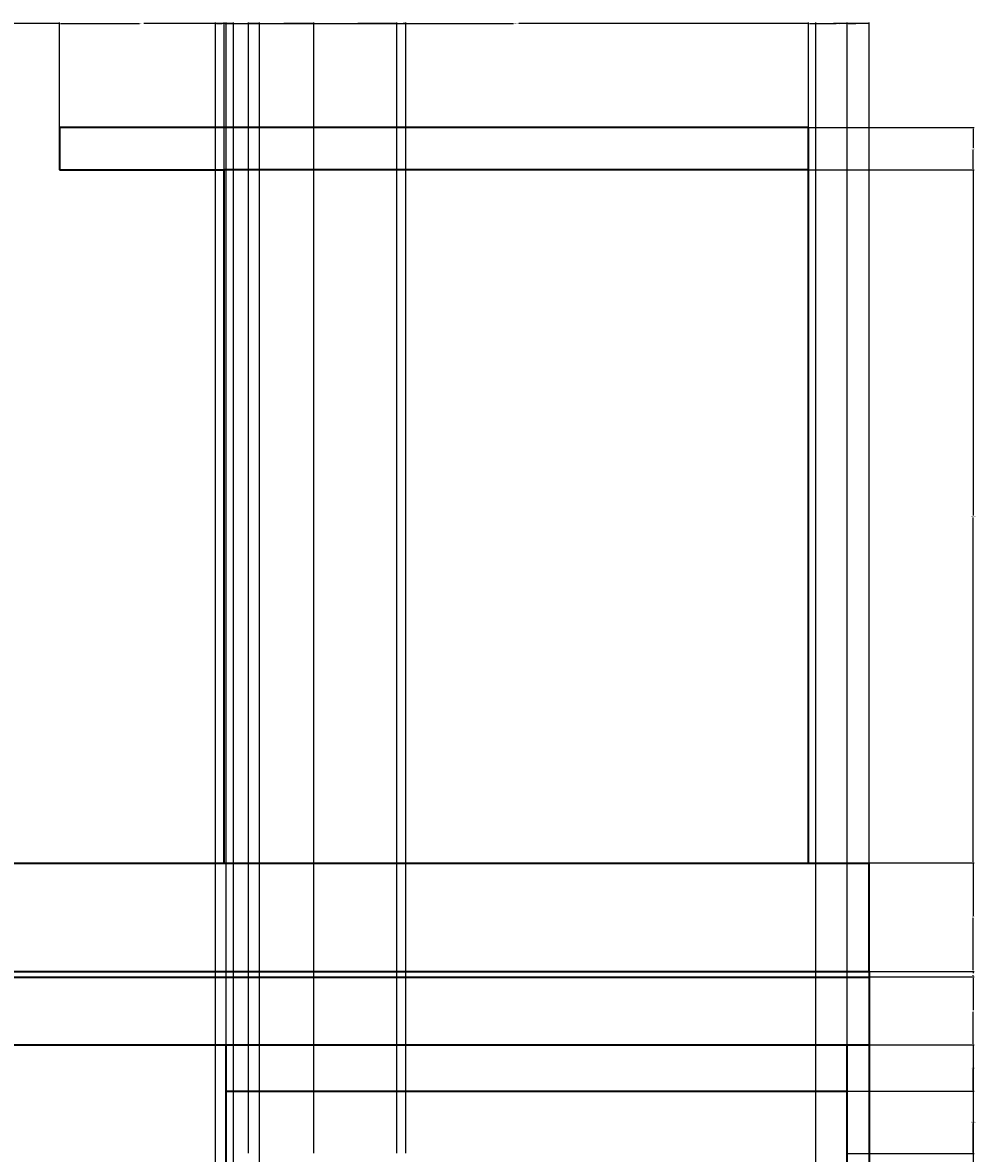
# Model space of a CAD drawing. Units: inches. Extents: x -7 to 391, y -12 to 303.
# Tile 5 of 5: x 222 to 391, y 103 to 303. Entities that reach past the tile are written whole.
import ezdxf

# ---------------------------------------------------------------- set-up
doc = ezdxf.new("R2010")
doc.units = ezdxf.units.IN
doc.header["$MEASUREMENT"] = 0
doc.layers.add('A-ANNO-DIMS', color=2, linetype='Continuous', lineweight=18)
doc.layers.add('A-ELEV', color=7, linetype='Continuous', lineweight=35)
doc.styles.get("Standard").update_dxf_attribs({"font": 'arial.ttf'})
doc.dimstyles.get("Standard").update_dxf_attribs({"dimtxt": 0.18, "dimasz": 0.18, "dimexe": 0.18, "dimexo": 0.0625, "dimgap": 0.09, "dimtad": 0, "dimtih": 1, "dimtoh": 1, "dimdec": 4, "dimzin": 0, "dimdsep": 46, "dimtxsty": 'Standard', "dimcen": 0.09, "dimadec": 0, "dimazin": 0, "dimtfac": 1, "dimtdec": 4, "dimtofl": 0, "dimtmove": 0, "dimatfit": 3, "dimfxl": 1, "dimtolj": 1, "dimtzin": 0, "dimarcsym": 0})

# ---------------------------------------------------------------- blocks, each defined once
blk = doc.blocks.new('*D1')
at = {"layer": 'A-ANNO-DIMS', "color": 0, "lineweight": -2, "transparency": 16777216}
for p, q in [((372.08, 122.18), (390.6, 122.18)), ((390.42, 122), (390.42, 64.44)), ((390.42, 6.53), (390.42, 64.08)), ((150.31, 6.35), (390.6, 6.35))]:
    blk.add_line(p, q, dxfattribs=at)
at = {"layer": 'A-ANNO-DIMS', "color": 0, "transparency": 16777216}
for points in [[(390.39, 122), (390.45, 122), (390.42, 122.18)], [(390.39, 6.53), (390.45, 6.53), (390.42, 6.35)]]:
    blk.add_solid(points, dxfattribs=at)
at = {"layer": 'Defpoints', "color": 0, "transparency": 16777216}
for p in [(372.02, 122.18), (390.42, 122.18), (150.24, 6.35)]:
    blk.add_point(p, dxfattribs=at)
at = {"layer": 'A-ANNO-DIMS', "color": 0, "transparency": 16777216, "insert": (390.42, 64.26), "char_height": 0.18, "attachment_point": 5}
blk.add_mtext('\\A1;115.83', dxfattribs=at)
blk = doc.blocks.new('*D2')
at = {"layer": 'A-ANNO-DIMS', "color": 0, "lineweight": -2, "transparency": 16777216}
for p, q in [((372.08, 134.18), (390.6, 134.18)), ((390.42, 134), (390.42, 128.36)), ((390.42, 122.36), (390.42, 128)), ((372.08, 122.18), (390.6, 122.18))]:
    blk.add_line(p, q, dxfattribs=at)
at = {"layer": 'A-ANNO-DIMS', "color": 0, "transparency": 16777216}
for points in [[(390.39, 134), (390.45, 134), (390.42, 134.18)], [(390.39, 122.36), (390.45, 122.36), (390.42, 122.18)]]:
    blk.add_solid(points, dxfattribs=at)
at = {"layer": 'Defpoints', "color": 0, "transparency": 16777216}
for p in [(372.02, 134.18), (390.42, 134.18), (372.02, 122.18)]:
    blk.add_point(p, dxfattribs=at)
at = {"layer": 'A-ANNO-DIMS', "color": 0, "transparency": 16777216, "insert": (390.42, 128.18), "char_height": 0.18, "attachment_point": 5}
blk.add_mtext('\\A1;12', dxfattribs=at)
blk = doc.blocks.new('*D3')
at = {"layer": 'A-ANNO-DIMS', "color": 0, "lineweight": -2, "transparency": 16777216}
for p, q in [((372.08, 135.18), (390.6, 135.18)), ((372.08, 134.18), (390.6, 134.18)), ((390.42, 135), (390.42, 134.86)), ((390.42, 134.36), (390.42, 134.5))]:
    blk.add_line(p, q, dxfattribs=at)
at = {"layer": 'A-ANNO-DIMS', "color": 0, "transparency": 16777216}
for points in [[(390.39, 135), (390.45, 135), (390.42, 135.18)], [(390.39, 134.36), (390.45, 134.36), (390.42, 134.18)]]:
    blk.add_solid(points, dxfattribs=at)
at = {"layer": 'Defpoints', "color": 0, "transparency": 16777216}
for p in [(372.02, 135.18), (372.02, 134.18), (390.42, 135.18)]:
    blk.add_point(p, dxfattribs=at)
at = {"layer": 'A-ANNO-DIMS', "color": 0, "transparency": 16777216, "insert": (390.42, 134.68), "char_height": 0.18, "attachment_point": 5}
blk.add_mtext('\\A1;1', dxfattribs=at)
blk = doc.blocks.new('*D4')
at = {"layer": 'A-ANNO-DIMS', "color": 0, "lineweight": -2, "transparency": 16777216}
for p, q in [((372.08, 154.35), (390.6, 154.35)), ((390.42, 154.17), (390.42, 144.94)), ((390.42, 135.36), (390.42, 144.58)), ((372.08, 135.18), (390.6, 135.18))]:
    blk.add_line(p, q, dxfattribs=at)
at = {"layer": 'A-ANNO-DIMS', "color": 0, "transparency": 16777216}
for points in [[(390.39, 154.17), (390.45, 154.17), (390.42, 154.35)], [(390.39, 135.36), (390.45, 135.36), (390.42, 135.18)]]:
    blk.add_solid(points, dxfattribs=at)
at = {"layer": 'Defpoints', "color": 0, "transparency": 16777216}
for p in [(372.02, 154.35), (390.42, 154.35), (372.02, 135.18)]:
    blk.add_point(p, dxfattribs=at)
at = {"layer": 'A-ANNO-DIMS', "color": 0, "transparency": 16777216, "insert": (390.42, 144.76), "char_height": 0.18, "attachment_point": 5}
blk.add_mtext('\\A1;19.17', dxfattribs=at)
blk = doc.blocks.new('*D5')
at = {"layer": 'A-ANNO-DIMS', "color": 0, "lineweight": -2, "transparency": 16777216}
for p, q in [((361.32, 276.97), (390.6, 276.97)), ((390.42, 276.79), (390.42, 215.84)), ((390.42, 154.53), (390.42, 215.47)), ((372.08, 154.35), (390.6, 154.35))]:
    blk.add_line(p, q, dxfattribs=at)
at = {"layer": 'A-ANNO-DIMS', "color": 0, "transparency": 16777216}
for points in [[(390.39, 276.79), (390.45, 276.79), (390.42, 276.97)], [(390.39, 154.53), (390.45, 154.53), (390.42, 154.35)]]:
    blk.add_solid(points, dxfattribs=at)
at = {"layer": 'Defpoints', "color": 0, "transparency": 16777216}
for p in [(361.25, 276.97), (390.42, 276.97), (372.02, 154.35)]:
    blk.add_point(p, dxfattribs=at)
at = {"layer": 'A-ANNO-DIMS', "color": 0, "transparency": 16777216, "insert": (390.42, 215.66), "char_height": 0.18, "attachment_point": 5}
blk.add_mtext('\\A1;122.62', dxfattribs=at)
blk = doc.blocks.new('*D6')
at = {"layer": 'A-ANNO-DIMS', "color": 0, "lineweight": -2, "transparency": 16777216}
for p, q in [((361.32, 284.43), (390.6, 284.43)), ((390.42, 284.25), (390.42, 280.88)), ((390.42, 277.15), (390.42, 280.52)), ((361.32, 276.97), (390.6, 276.97))]:
    blk.add_line(p, q, dxfattribs=at)
at = {"layer": 'A-ANNO-DIMS', "color": 0, "transparency": 16777216}
for points in [[(390.39, 284.25), (390.45, 284.25), (390.42, 284.43)], [(390.39, 277.15), (390.45, 277.15), (390.42, 276.97)]]:
    blk.add_solid(points, dxfattribs=at)
at = {"layer": 'Defpoints', "color": 0, "transparency": 16777216}
for p in [(361.25, 284.43), (390.42, 284.43), (361.25, 276.97)]:
    blk.add_point(p, dxfattribs=at)
at = {"layer": 'A-ANNO-DIMS', "color": 0, "transparency": 16777216, "insert": (390.42, 280.7), "char_height": 0.18, "attachment_point": 5}
blk.add_mtext('\\A1;7.465', dxfattribs=at)
blk = doc.blocks.new('*D21')
at = {"layer": 'A-ANNO-DIMS', "color": 0, "lineweight": -2, "transparency": 16777216}
for p, q in [((138.24, 134.24), (138.24, 303.01)), ((138.42, 302.83), (183.11, 302.83)), ((228.58, 302.83), (183.89, 302.83)), ((228.76, 284.49), (228.76, 303.01))]:
    blk.add_line(p, q, dxfattribs=at)
at = {"layer": 'A-ANNO-DIMS', "color": 0, "transparency": 16777216}
for points in [[(138.42, 302.86), (138.42, 302.8), (138.24, 302.83)], [(228.58, 302.86), (228.58, 302.8), (228.76, 302.83)]]:
    blk.add_solid(points, dxfattribs=at)
at = {"layer": 'Defpoints', "color": 0, "transparency": 16777216}
for p in [(228.76, 302.83), (228.76, 284.43), (138.24, 134.18)]:
    blk.add_point(p, dxfattribs=at)
at = {"layer": 'A-ANNO-DIMS', "color": 0, "transparency": 16777216, "insert": (183.5, 302.83), "char_height": 0.18, "attachment_point": 5}
blk.add_mtext('\\A1;90.52', dxfattribs=at)
blk = doc.blocks.new('*D22')
at = {"layer": 'A-ANNO-DIMS', "color": 0, "lineweight": -2, "transparency": 16777216}
for p, q in [((228.76, 284.49), (228.76, 303.01)), ((228.94, 302.83), (242.93, 302.83)), ((257.69, 302.83), (243.69, 302.83)), ((257.87, 277.03), (257.87, 303.01))]:
    blk.add_line(p, q, dxfattribs=at)
at = {"layer": 'A-ANNO-DIMS', "color": 0, "transparency": 16777216}
for points in [[(228.94, 302.86), (228.94, 302.8), (228.76, 302.83)], [(257.69, 302.86), (257.69, 302.8), (257.87, 302.83)]]:
    blk.add_solid(points, dxfattribs=at)
at = {"layer": 'Defpoints', "color": 0, "transparency": 16777216}
for p in [(257.87, 302.83), (228.76, 284.43), (257.87, 276.97)]:
    blk.add_point(p, dxfattribs=at)
at = {"layer": 'A-ANNO-DIMS', "color": 0, "transparency": 16777216, "insert": (243.31, 302.83), "char_height": 0.18, "attachment_point": 5}
blk.add_mtext('\\A1;29.11', dxfattribs=at)
blk = doc.blocks.new('*D23')
at = {"layer": 'A-ANNO-DIMS', "color": 0, "lineweight": -2, "transparency": 16777216}
for p, q in [((257.87, 277.03), (257.87, 303.01)), ((258.05, 302.83), (309.1, 302.83)), ((361.07, 302.83), (310.02, 302.83)), ((361.25, 284.49), (361.25, 303.01))]:
    blk.add_line(p, q, dxfattribs=at)
at = {"layer": 'A-ANNO-DIMS', "color": 0, "transparency": 16777216}
for points in [[(258.05, 302.86), (258.05, 302.8), (257.87, 302.83)], [(361.07, 302.86), (361.07, 302.8), (361.25, 302.83)]]:
    blk.add_solid(points, dxfattribs=at)
at = {"layer": 'Defpoints', "color": 0, "transparency": 16777216}
for p in [(361.25, 302.83), (361.25, 284.43), (257.87, 276.97)]:
    blk.add_point(p, dxfattribs=at)
at = {"layer": 'A-ANNO-DIMS', "color": 0, "transparency": 16777216, "insert": (309.56, 302.83), "char_height": 0.18, "attachment_point": 5}
blk.add_mtext('\\A1;103.39', dxfattribs=at)
blk = doc.blocks.new('*D24')
at = {"layer": 'A-ANNO-DIMS', "color": 0, "lineweight": -2, "transparency": 16777216}
for p, q in [((361.25, 284.49), (361.25, 303.01)), ((361.43, 302.83), (366.18, 302.83)), ((371.84, 302.83), (367.09, 302.83)), ((372.02, 154.41), (372.02, 303.01))]:
    blk.add_line(p, q, dxfattribs=at)
at = {"layer": 'A-ANNO-DIMS', "color": 0, "transparency": 16777216}
for points in [[(361.43, 302.86), (361.43, 302.8), (361.25, 302.83)], [(371.84, 302.86), (371.84, 302.8), (372.02, 302.83)]]:
    blk.add_solid(points, dxfattribs=at)
at = {"layer": 'Defpoints', "color": 0, "transparency": 16777216}
for p in [(372.02, 302.83), (361.25, 284.43), (372.02, 154.35)]:
    blk.add_point(p, dxfattribs=at)
at = {"layer": 'A-ANNO-DIMS', "color": 0, "transparency": 16777216, "insert": (366.64, 302.83), "char_height": 0.18, "attachment_point": 5}
blk.add_mtext('\\A1;10.767', dxfattribs=at)
blk = doc.blocks.new('*D39')
at = {"layer": 'A-ANNO-DIMS', "color": 0, "lineweight": -2, "transparency": 16777216}
for p, q in [((372.02, 154.28), (372.02, -12.23)), ((246.74, 6.28), (246.74, -12.23)), ((246.92, -12.05), (308.92, -12.05)), ((371.84, -12.05), (309.84, -12.05))]:
    blk.add_line(p, q, dxfattribs=at)
at = {"layer": 'A-ANNO-DIMS', "color": 0, "transparency": 16777216}
for points in [[(246.92, -12.02), (246.92, -12.08), (246.74, -12.05)], [(371.84, -12.02), (371.84, -12.08), (372.02, -12.05)]]:
    blk.add_solid(points, dxfattribs=at)
at = {"layer": 'Defpoints', "color": 0, "transparency": 16777216}
for p in [(372.02, 154.35), (246.74, 6.35), (372.02, -12.05)]:
    blk.add_point(p, dxfattribs=at)
at = {"layer": 'A-ANNO-DIMS', "color": 0, "transparency": 16777216, "insert": (309.38, -12.05), "char_height": 0.18, "attachment_point": 5}
blk.add_mtext('\\A1;125.28', dxfattribs=at)
blk = doc.blocks.new('*D46')
at = {"layer": 'A-ANNO-DIMS', "color": 0, "lineweight": -2, "transparency": 16777216}
for p, q in [((256.34, 96.52), (256.34, 303.01)), ((256.52, 302.83), (257.55, 302.83)), ((259.37, 302.83), (258.34, 302.83)), ((259.55, 96.52), (259.55, 303.01))]:
    blk.add_line(p, q, dxfattribs=at)
at = {"layer": 'A-ANNO-DIMS', "color": 0, "transparency": 16777216}
for points in [[(256.52, 302.86), (256.52, 302.8), (256.34, 302.83)], [(259.37, 302.86), (259.37, 302.8), (259.55, 302.83)]]:
    blk.add_solid(points, dxfattribs=at)
at = {"layer": 'Defpoints', "color": 0, "transparency": 16777216}
for p in [(259.55, 302.83), (256.34, 96.46), (259.55, 96.46)]:
    blk.add_point(p, dxfattribs=at)
at = {"layer": 'A-ANNO-DIMS', "color": 0, "transparency": 16777216, "insert": (257.95, 302.83), "char_height": 0.18, "attachment_point": 5}
blk.add_mtext('\\A1;3.217', dxfattribs=at)
blk = doc.blocks.new('*D47')
at = {"layer": 'A-ANNO-DIMS', "color": 0, "lineweight": -2, "transparency": 16777216}
for p, q in [((259.55, 96.52), (259.55, 303.01)), ((259.73, 302.83), (261.45, 302.83)), ((263.95, 302.83), (262.24, 302.83)), ((264.13, 96.52), (264.13, 303.01))]:
    blk.add_line(p, q, dxfattribs=at)
at = {"layer": 'A-ANNO-DIMS', "color": 0, "transparency": 16777216}
for points in [[(259.73, 302.86), (259.73, 302.8), (259.55, 302.83)], [(263.95, 302.86), (263.95, 302.8), (264.13, 302.83)]]:
    blk.add_solid(points, dxfattribs=at)
at = {"layer": 'Defpoints', "color": 0, "transparency": 16777216}
for p in [(264.13, 302.83), (259.55, 96.46), (264.13, 96.46)]:
    blk.add_point(p, dxfattribs=at)
at = {"layer": 'A-ANNO-DIMS', "color": 0, "transparency": 16777216, "insert": (261.84, 302.83), "char_height": 0.18, "attachment_point": 5}
blk.add_mtext('\\A1;4.579', dxfattribs=at)
blk = doc.blocks.new('*D51')
at = {"layer": 'A-ANNO-DIMS', "color": 0, "lineweight": -2, "transparency": 16777216}
for p, q in [((362.55, 96.52), (362.55, 303.01)), ((362.73, 302.83), (364.93, 302.83)), ((367.92, 302.83), (365.72, 302.83)), ((368.1, 103.04), (368.1, 303.01))]:
    blk.add_line(p, q, dxfattribs=at)
at = {"layer": 'A-ANNO-DIMS', "color": 0, "transparency": 16777216}
for points in [[(362.73, 302.86), (362.73, 302.8), (362.55, 302.83)], [(367.92, 302.86), (367.92, 302.8), (368.1, 302.83)]]:
    blk.add_solid(points, dxfattribs=at)
at = {"layer": 'Defpoints', "color": 0, "transparency": 16777216}
for p in [(368.1, 302.83), (368.1, 102.98), (362.55, 96.46)]:
    blk.add_point(p, dxfattribs=at)
at = {"layer": 'A-ANNO-DIMS', "color": 0, "transparency": 16777216, "insert": (365.32, 302.83), "char_height": 0.18, "attachment_point": 5}
blk.add_mtext('\\A1;5.549', dxfattribs=at)
blk = doc.blocks.new('*D52')
at = {"layer": 'A-ANNO-DIMS', "color": 0, "lineweight": -2, "transparency": 16777216}
for p, q in [((368.1, 103.04), (368.1, 303.01)), ((368.28, 302.83), (369.67, 302.83)), ((371.84, 302.83), (370.45, 302.83)), ((372.02, 122.24), (372.02, 303.01))]:
    blk.add_line(p, q, dxfattribs=at)
at = {"layer": 'A-ANNO-DIMS', "color": 0, "transparency": 16777216}
for points in [[(368.28, 302.86), (368.28, 302.8), (368.1, 302.83)], [(371.84, 302.86), (371.84, 302.8), (372.02, 302.83)]]:
    blk.add_solid(points, dxfattribs=at)
at = {"layer": 'Defpoints', "color": 0, "transparency": 16777216}
for p in [(372.02, 302.83), (372.02, 122.18), (368.1, 102.98)]:
    blk.add_point(p, dxfattribs=at)
at = {"layer": 'A-ANNO-DIMS', "color": 0, "transparency": 16777216, "insert": (370.06, 302.83), "char_height": 0.18, "attachment_point": 5}
blk.add_mtext('\\A1;3.922', dxfattribs=at)
blk = doc.blocks.new('*D53')
at = {"layer": 'A-ANNO-DIMS', "color": 0, "lineweight": -2, "transparency": 16777216}
for p, q in [((256.34, 96.52), (256.34, 303.01)), ((256.52, 302.83), (256.92, 302.83)), ((258.09, 302.83), (257.69, 302.83)), ((258.27, 103.04), (258.27, 303.01))]:
    blk.add_line(p, q, dxfattribs=at)
at = {"layer": 'A-ANNO-DIMS', "color": 0, "transparency": 16777216}
for points in [[(256.52, 302.86), (256.52, 302.8), (256.34, 302.83)], [(258.09, 302.86), (258.09, 302.8), (258.27, 302.83)]]:
    blk.add_solid(points, dxfattribs=at)
at = {"layer": 'Defpoints', "color": 0, "transparency": 16777216}
for p in [(258.27, 302.83), (258.27, 102.98), (256.34, 96.46)]:
    blk.add_point(p, dxfattribs=at)
at = {"layer": 'A-ANNO-DIMS', "color": 0, "transparency": 16777216, "insert": (257.3, 302.83), "char_height": 0.18, "attachment_point": 5}
blk.add_mtext('\\A1;1.933', dxfattribs=at)
blk = doc.blocks.new('*D54')
at = {"layer": 'A-ANNO-DIMS', "color": 0, "lineweight": -2, "transparency": 16777216}
for p, q in [((262.22, 103.04), (262.22, 303.01)), ((262.4, 302.83), (267.53, 302.83)), ((273.57, 302.83), (268.44, 302.83)), ((273.75, 103.04), (273.75, 303.01))]:
    blk.add_line(p, q, dxfattribs=at)
at = {"layer": 'A-ANNO-DIMS', "color": 0, "transparency": 16777216}
for points in [[(262.4, 302.86), (262.4, 302.8), (262.22, 302.83)], [(273.57, 302.86), (273.57, 302.8), (273.75, 302.83)]]:
    blk.add_solid(points, dxfattribs=at)
at = {"layer": 'Defpoints', "color": 0, "transparency": 16777216}
for p in [(273.75, 302.83), (262.22, 102.98), (273.75, 102.98)]:
    blk.add_point(p, dxfattribs=at)
at = {"layer": 'A-ANNO-DIMS', "color": 0, "transparency": 16777216, "insert": (267.99, 302.83), "char_height": 0.18, "attachment_point": 5}
blk.add_mtext('\\A1;11.534', dxfattribs=at)
blk = doc.blocks.new('*D55')
at = {"layer": 'A-ANNO-DIMS', "color": 0, "lineweight": -2, "transparency": 16777216}
for p, q in [((273.75, 103.04), (273.75, 303.01)), ((273.93, 302.83), (280.65, 302.83)), ((288.28, 302.83), (281.56, 302.83)), ((288.46, 103.04), (288.46, 303.01))]:
    blk.add_line(p, q, dxfattribs=at)
at = {"layer": 'A-ANNO-DIMS', "color": 0, "transparency": 16777216}
for points in [[(273.93, 302.86), (273.93, 302.8), (273.75, 302.83)], [(288.28, 302.86), (288.28, 302.8), (288.46, 302.83)]]:
    blk.add_solid(points, dxfattribs=at)
at = {"layer": 'Defpoints', "color": 0, "transparency": 16777216}
for p in [(288.46, 302.83), (273.75, 102.98), (288.46, 102.98)]:
    blk.add_point(p, dxfattribs=at)
at = {"layer": 'A-ANNO-DIMS', "color": 0, "transparency": 16777216, "insert": (281.11, 302.83), "char_height": 0.18, "attachment_point": 5}
blk.add_mtext('\\A1;14.706', dxfattribs=at)
blk = doc.blocks.new('*D56')
at = {"layer": 'A-ANNO-DIMS', "color": 0, "lineweight": -2, "transparency": 16777216}
for p, q in [((288.46, 103.04), (288.46, 303.01)), ((288.64, 302.83), (288.93, 302.83)), ((289.85, 302.83), (289.56, 302.83)), ((290.03, 103.04), (290.03, 303.01))]:
    blk.add_line(p, q, dxfattribs=at)
at = {"layer": 'A-ANNO-DIMS', "color": 0, "transparency": 16777216}
for points in [[(288.64, 302.86), (288.64, 302.8), (288.46, 302.83)], [(289.85, 302.86), (289.85, 302.8), (290.03, 302.83)]]:
    blk.add_solid(points, dxfattribs=at)
at = {"layer": 'Defpoints', "color": 0, "transparency": 16777216}
for p in [(290.03, 302.83), (288.46, 102.98), (290.03, 102.98)]:
    blk.add_point(p, dxfattribs=at)
at = {"layer": 'A-ANNO-DIMS', "color": 0, "transparency": 16777216, "insert": (289.24, 302.83), "char_height": 0.18, "attachment_point": 5}
blk.add_mtext('\\A1;1.57', dxfattribs=at)
blk = doc.blocks.new('*D61')
at = {"layer": 'A-ANNO-DIMS', "color": 0, "lineweight": -2, "transparency": 16777216}
for p, q in [((368.16, 102.98), (390.6, 102.98)), ((390.42, 102.8), (390.42, 99.9)), ((390.42, 96.64), (390.42, 99.53)), ((372.08, 96.46), (390.6, 96.46))]:
    blk.add_line(p, q, dxfattribs=at)
at = {"layer": 'A-ANNO-DIMS', "color": 0, "transparency": 16777216}
for points in [[(390.39, 102.8), (390.45, 102.8), (390.42, 102.98)], [(390.39, 96.64), (390.45, 96.64), (390.42, 96.46)]]:
    blk.add_solid(points, dxfattribs=at)
at = {"layer": 'Defpoints', "color": 0, "transparency": 16777216}
for p in [(368.1, 102.98), (390.42, 102.98), (372.02, 96.46)]:
    blk.add_point(p, dxfattribs=at)
at = {"layer": 'A-ANNO-DIMS', "color": 0, "transparency": 16777216, "insert": (390.42, 99.72), "char_height": 0.18, "attachment_point": 5}
blk.add_mtext('\\A1;6.52', dxfattribs=at)
blk = doc.blocks.new('*D62')
at = {"layer": 'A-ANNO-DIMS', "color": 0, "lineweight": -2, "transparency": 16777216}
for p, q in [((368.16, 113.96), (390.6, 113.96)), ((390.42, 113.78), (390.42, 108.65)), ((390.42, 103.16), (390.42, 108.29)), ((368.16, 102.98), (390.6, 102.98))]:
    blk.add_line(p, q, dxfattribs=at)
at = {"layer": 'A-ANNO-DIMS', "color": 0, "transparency": 16777216}
for points in [[(390.39, 113.78), (390.45, 113.78), (390.42, 113.96)], [(390.39, 103.16), (390.45, 103.16), (390.42, 102.98)]]:
    blk.add_solid(points, dxfattribs=at)
at = {"layer": 'Defpoints', "color": 0, "transparency": 16777216}
for p in [(368.1, 113.96), (390.42, 113.96), (368.1, 102.98)]:
    blk.add_point(p, dxfattribs=at)
at = {"layer": 'A-ANNO-DIMS', "color": 0, "transparency": 16777216, "insert": (390.42, 108.47), "char_height": 0.18, "attachment_point": 5}
blk.add_mtext('\\A1;10.988', dxfattribs=at)
blk = doc.blocks.new('*D63')
at = {"layer": 'A-ANNO-DIMS', "color": 0, "lineweight": -2, "transparency": 16777216}
for p, q in [((372.08, 122.18), (390.6, 122.18)), ((390.42, 122), (390.42, 118.25)), ((390.42, 114.14), (390.42, 117.89)), ((368.16, 113.96), (390.6, 113.96))]:
    blk.add_line(p, q, dxfattribs=at)
at = {"layer": 'A-ANNO-DIMS', "color": 0, "transparency": 16777216}
for points in [[(390.39, 122), (390.45, 122), (390.42, 122.18)], [(390.39, 114.14), (390.45, 114.14), (390.42, 113.96)]]:
    blk.add_solid(points, dxfattribs=at)
at = {"layer": 'Defpoints', "color": 0, "transparency": 16777216}
for p in [(372.02, 122.18), (390.42, 122.18), (368.1, 113.96)]:
    blk.add_point(p, dxfattribs=at)
at = {"layer": 'A-ANNO-DIMS', "color": 0, "transparency": 16777216, "insert": (390.42, 118.07), "char_height": 0.18, "attachment_point": 5}
blk.add_mtext('\\A1;8.213', dxfattribs=at)

msp = doc.modelspace()

# ---------------------------------------------------------------- linework, layer by layer
at = {"layer": 'A-ELEV'}
for p, q in [((257.8665, 284.432), (228.758, 284.432)), ((228.758, 284.432), (228.758, 276.9675)), ((361.2537, 284.432), (257.8665, 284.432)), ((361.2537, 154.3452), (361.2537, 284.432)), ((228.758, 276.9675), (257.8665, 276.9675)), ((257.8665, 276.9675), (257.8665, 154.3452)), ((361.2537, 276.9675), (257.8665, 276.9675)), ((15.8204, 154.3452), (372.0212, 154.3452)), ((372.0212, 135.1767), (372.0212, 154.3452)), ((137.2426, 135.1767), (372.0212, 135.1767)), ((138.2426, 134.1767), (372.0212, 134.1767)), ((372.0212, 135.1767), (372.0212, 6.3452)), ((150.2426, 122.1767), (372.0212, 122.1767)), ((258.2707, 96.456), (258.2707, 122.1767)), ((368.0993, 96.456), (368.0993, 122.1767)), ((258.2707, 113.9639), (368.0993, 113.9639))]:
    msp.add_line(p, q, dxfattribs=at)

# ---------------------------------------------------------------- dimensions: what is measured, and where the dimension line sits
at = {"layer": 'A-ANNO-DIMS'}
for base, p1, p2, override, picture, middle in [((228.758, 302.832), (138.2426, 134.1767), (228.758, 284.432), {"dimdec": 2, "dimlfac": 1, "dimrnd": 0, "dimzin": 0, "dimdsep": 46, "dimlunit": 2}, '*D21', (183.5003, 302.832)), ((257.8665, 302.832), (228.758, 284.432), (257.8665, 276.9675), {"dimdec": 2, "dimlfac": 1, "dimrnd": 0, "dimzin": 0, "dimdsep": 46, "dimlunit": 2}, '*D22', (243.3122, 302.832)), ((259.5545, 302.832), (256.3377, 96.456), (259.5545, 96.456), {"dimdec": 3, "dimlfac": 1, "dimrnd": 0, "dimzin": 0, "dimdsep": 46, "dimlunit": 2}, '*D46', (257.9461, 302.832)), ((258.2707, 302.832), (256.3377, 96.456), (258.2707, 102.9762), {"dimdec": 3, "dimlfac": 1, "dimrnd": 0, "dimzin": 0, "dimdsep": 46, "dimlunit": 2}, '*D53', (257.3042, 302.832)), ((361.2537, 302.832), (257.8665, 276.9675), (361.2537, 284.432), {"dimdec": 2, "dimlfac": 1, "dimrnd": 0, "dimzin": 0, "dimdsep": 46, "dimlunit": 2}, '*D23', (309.5601, 302.832)), ((264.1332, 302.832), (259.5545, 96.456), (264.1332, 96.456), {"dimdec": 3, "dimlfac": 1, "dimrnd": 0, "dimzin": 0, "dimdsep": 46, "dimlunit": 2}, '*D47', (261.8439, 302.832)), ((273.7532, 302.832), (262.2191, 102.9762), (273.7532, 102.9762), {"dimdec": 3, "dimlfac": 1, "dimrnd": 0, "dimzin": 0, "dimdsep": 46, "dimlunit": 2}, '*D54', (267.9862, 302.832)), ((288.4588, 302.832), (273.7532, 102.9762), (288.4588, 102.9762), {"dimdec": 3, "dimlfac": 1, "dimrnd": 0, "dimzin": 0, "dimdsep": 46, "dimlunit": 2}, '*D55', (281.106, 302.832)), ((290.0289, 302.832), (288.4588, 102.9762), (290.0289, 102.9762), {"dimdec": 2, "dimlfac": 1, "dimrnd": 0, "dimzin": 0, "dimdsep": 46, "dimlunit": 2}, '*D56', (289.2439, 302.832)), ((372.02119, 302.83205), (361.2537, 284.43205), (372.02119, 154.34518), {"dimdec": 3, "dimlfac": 1, "dimrnd": 0, "dimzin": 0, "dimdsep": 46, "dimlunit": 2}, '*D24', (366.63744, 302.83205)), ((368.0993, 302.832), (362.5506, 96.456), (368.0993, 102.9762), {"dimdec": 3, "dimlfac": 1, "dimrnd": 0, "dimzin": 0, "dimdsep": 46, "dimlunit": 2}, '*D51', (365.325, 302.832)), ((372.0212, 302.832), (368.0993, 102.9762), (372.0212, 122.1767), {"dimdec": 3, "dimlfac": 1, "dimrnd": 0, "dimzin": 0, "dimdsep": 46, "dimlunit": 2}, '*D52', (370.0602, 302.832)), ((372.0212, -12.0548), (246.7395, 6.3452), (372.0212, 154.3452), {"dimdec": 2, "dimlfac": 1, "dimrnd": 0, "dimzin": 0, "dimdsep": 46, "dimlunit": 2}, '*D39', (309.3803, -12.0548))]:
    dim = msp.add_linear_dim(base=base, p1=p1, p2=p2, dimstyle='Standard', override=override, dxfattribs=at)
    dim.commit()
    dim.dimension.update_dxf_attribs({"geometry": picture, "text_midpoint": middle})
for base, p1, p2, override, picture, middle in [((390.42119, 284.43205), (361.2537, 276.96746), (361.2537, 284.43205), {"dimdec": 3, "dimlfac": 1, "dimrnd": 0, "dimzin": 0, "dimdsep": 46, "dimlunit": 2}, '*D6', (390.42119, 280.69976)), ((390.4212, 276.9675), (372.0212, 154.3452), (361.2537, 276.9675), {"dimdec": 2, "dimlfac": 1, "dimrnd": 0, "dimzin": 0, "dimdsep": 46, "dimlunit": 2}, '*D5', (390.4212, 215.6563)), ((390.4212, 154.3452), (372.0212, 135.1767), (372.0212, 154.3452), {"dimdec": 2, "dimlfac": 1, "dimrnd": 0, "dimzin": 0, "dimdsep": 46, "dimlunit": 2}, '*D4', (390.4212, 144.761)), ((390.4212, 135.1767), (372.0212, 134.1767), (372.0212, 135.1767), {"dimdec": 0, "dimlfac": 1, "dimrnd": 0, "dimzin": 0, "dimdsep": 46, "dimlunit": 2}, '*D3', (390.4212, 134.6767)), ((390.4212, 134.1767), (372.0212, 122.1767), (372.0212, 134.1767), {"dimdec": 0, "dimlfac": 1, "dimrnd": 0, "dimzin": 0, "dimdsep": 46, "dimlunit": 2}, '*D2', (390.4212, 128.1767)), ((390.4212, 122.1767), (150.2426, 6.3452), (372.0212, 122.1767), {"dimdec": 2, "dimlfac": 1, "dimrnd": 0, "dimzin": 0, "dimdsep": 46, "dimlunit": 2}, '*D1', (390.4212, 64.261)), ((390.4212, 122.1767), (368.0993, 113.9639), (372.0212, 122.1767), {"dimdec": 3, "dimlfac": 1, "dimrnd": 0, "dimzin": 0, "dimdsep": 46, "dimlunit": 2}, '*D63', (390.4212, 118.0703)), ((390.4212, 113.9639), (368.0993, 102.9762), (368.0993, 113.9639), {"dimdec": 3, "dimlfac": 1, "dimrnd": 0, "dimzin": 0, "dimdsep": 46, "dimlunit": 2}, '*D62', (390.4212, 108.4701)), ((390.4212, 102.9762), (372.0212, 96.456), (368.0993, 102.9762), {"dimdec": 2, "dimlfac": 1, "dimrnd": 0, "dimzin": 0, "dimdsep": 46, "dimlunit": 2}, '*D61', (390.4212, 99.7161))]:
    dim = msp.add_linear_dim(base=base, p1=p1, p2=p2, angle=90, dimstyle='Standard', override=override, dxfattribs=at)
    dim.commit()
    dim.dimension.update_dxf_attribs({"geometry": picture, "text_midpoint": middle})

doc.saveas('drawing.dxf')
